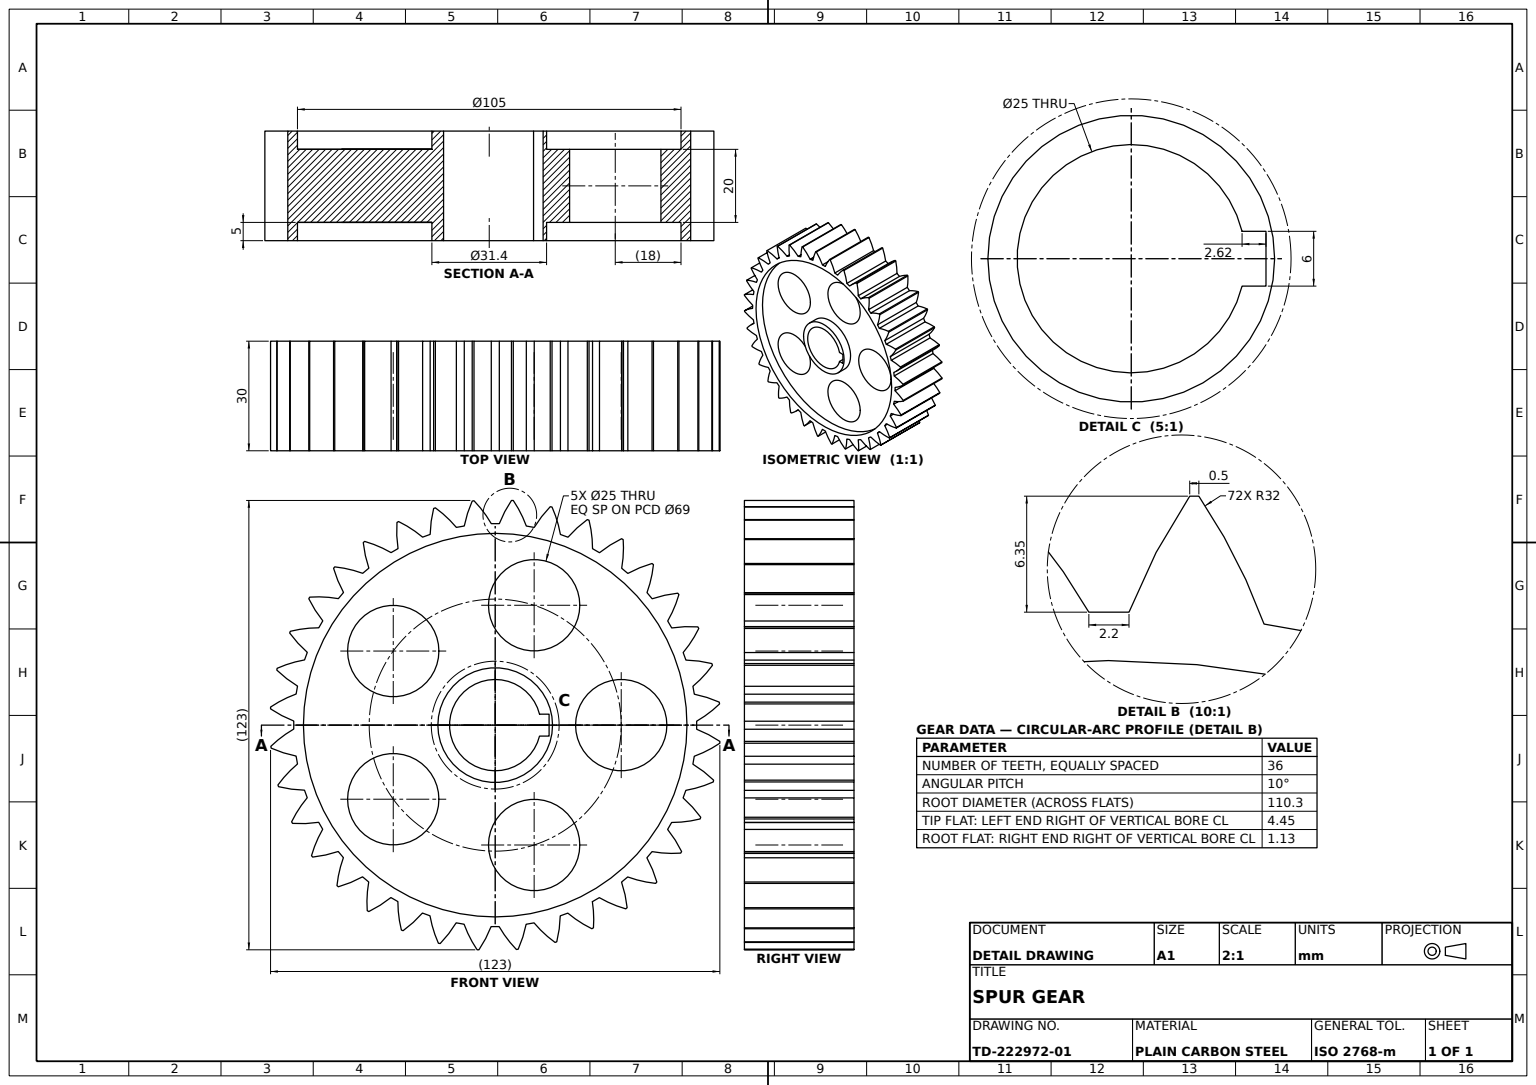
from build123d import *

# Parameters (mm, degrees)
GEAR_RIM_36T_DEPTH           = 15
SKETCH1_3_R                  = 52.5
GEAR_WEB_DEPTH               = 10
LIGHTENING_HOLES_SKETCH_R    = 12.5
LIGHTENING_HOLES_5X_18_DEPTH = 20
HUB_SKETCH_R                 = 15.7
HUB_DEPTH                    = 15
KEYED_BORE_DEPTH             = 30


with BuildPart() as part:
    # Gear Profile Sketch 36T → Gear Rim 36T (new, symmetric)
    with BuildSketch(Plane(origin=(0, 0, 0), x_dir=(1, 0, 0), z_dir=(0, 1, 0))):
        with BuildLine():
            Line((4.95, 61.5), (4.45, 61.5))
            ThreePointArc((4.45, 61.5), (2.609142561, 58.418391887), (1.125, 55.15))
            Line((1.125, 55.15), (0, 55.15))
            Line((0, 55.15), (-1.073339337, 55.15))
            ThreePointArc((-1.073339337, 55.15), (-3.245576648, 58.433413305), (-5.804564549, 61.42523529))
            Line((-5.804564549, 61.42523529), (-6.296968426, 61.338411201))
            ThreePointArc((-6.296968426, 61.338411201), (-7.574743471, 57.9839581), (-8.468788276, 54.507501778))
            Line((-8.468788276, 54.507501778), (-10.633729899, 54.125764159))
            ThreePointArc((-10.633729899, 54.125764159), (-13.343124781, 56.982089988), (-16.382760342, 59.484095888))
            Line((-16.382760342, 59.484095888), (-16.852606652, 59.313085816))
            ThreePointArc((-16.852606652, 59.313085816), (-17.528474755, 55.787711087), (-17.805256706, 52.208820698))
            Line((-17.805256706, 52.208820698), (-19.871019959, 51.456944362))
            ThreePointArc((-19.871019959, 51.456944362), (-23.03524882, 53.7993947), (-26.463174251, 55.735562333))
            Line((-26.463174251, 55.735562333), (-26.896186953, 55.485562333))
            ThreePointArc((-26.896186953, 55.485562333), (-26.949612204, 51.896382703), (-26.600721421, 48.323801019))
            Line((-26.600721421, 48.323801019), (-28.504539133, 47.22463135))
            ThreePointArc((-28.504539133, 47.22463135), (-32.02745848, 48.982032028), (-35.739518002, 50.29353192))
            Line((-35.739518002, 50.29353192), (-36.122540224, 49.972138115))
            ThreePointArc((-36.122540224, 49.972138115), (-35.551899323, 46.428208991), (-34.587936676, 42.970487099))
            Line((-34.587936676, 42.970487099), (-36.271962309, 41.557421811))
            ThreePointArc((-36.271962309, 41.557421811), (-40.04653002, 42.676375099), (-43.929934584, 43.323357989))
            Line((-43.929934584, 43.323357989), (-44.251328389, 42.940335768))
            ThreePointArc((-44.251328389, 42.940335768), (-43.073959971, 39.549337643), (-41.524214977, 36.311536673))
            Line((-41.524214977, 36.311536673), (-42.937280265, 34.627511039))
            ThreePointArc((-42.937280265, 34.627511039), (-46.84880801, 35.074018108), (-50.785562333, 35.036825749))
            Line((-50.785562333, 35.036825749), (-51.035562333, 34.603813047))
            ThreePointArc((-51.035562333, 34.603813047), (-49.287240142, 31.468779683), (-47.198801019, 28.549278579))
            Line((-47.198801019, 28.549278579), (-48.297970687, 26.645460867))
            ThreePointArc((-48.297970687, 26.645460867), (-52.227608676, 26.405954826), (-56.098096469, 25.685717287))
            Line((-56.098096469, 25.685717287), (-56.269106541, 25.215870977))
            ThreePointArc((-56.269106541, 25.215870977), (-54.002952462, 22.432058777), (-51.439275375, 19.919565103))
            Line((-51.439275375, 19.919565103), (-52.19115171, 17.853801849))
            ThreePointArc((-52.19115171, 17.853801849), (-56.01949988, 16.935559967), (-59.706118331, 15.554161304))
            Line((-59.706118331, 15.554161304), (-59.79294242, 15.061757427))
            ThreePointArc((-59.79294242, 15.061757427), (-57.077812398, 12.713751116), (-54.116793379, 10.68460572))
            Line((-54.116793379, 10.68460572), (-54.498530999, 8.519664097))
            ThreePointArc((-54.498530999, 8.519664097), (-58.109266928, 6.950586689), (-61.5, 4.95))
            Line((-61.5, 4.95), (-61.5, 4.45))
            ThreePointArc((-61.5, 4.45), (-58.418391887, 2.609142561), (-55.15, 1.125))
            Line((-55.15, 1.125), (-55.15, -1.073339337))
            ThreePointArc((-55.15, -1.073339337), (-58.433413305, -3.245576648), (-61.42523529, -5.804564549))
            Line((-61.42523529, -5.804564549), (-61.338411201, -6.296968426))
            ThreePointArc((-61.338411201, -6.296968426), (-57.9839581, -7.574743471), (-54.507501778, -8.468788276))
            Line((-54.507501778, -8.468788276), (-54.125764159, -10.633729899))
            ThreePointArc((-54.125764159, -10.633729899), (-56.982089988, -13.343124781), (-59.484095888, -16.382760342))
            Line((-59.484095888, -16.382760342), (-59.313085816, -16.852606652))
            ThreePointArc((-59.313085816, -16.852606652), (-55.787711087, -17.528474755), (-52.208820698, -17.805256706))
            Line((-52.208820698, -17.805256706), (-51.456944362, -19.871019959))
            ThreePointArc((-51.456944362, -19.871019959), (-53.7993947, -23.03524882), (-55.735562333, -26.463174251))
            Line((-55.735562333, -26.463174251), (-55.485562333, -26.896186953))
            ThreePointArc((-55.485562333, -26.896186953), (-51.896382703, -26.949612204), (-48.323801019, -26.600721421))
            Line((-48.323801019, -26.600721421), (-47.22463135, -28.504539133))
            ThreePointArc((-47.22463135, -28.504539133), (-48.982032028, -32.02745848), (-50.29353192, -35.739518002))
            Line((-50.29353192, -35.739518002), (-49.972138115, -36.122540224))
            ThreePointArc((-49.972138115, -36.122540224), (-46.428208991, -35.551899323), (-42.970487099, -34.587936676))
            Line((-42.970487099, -34.587936676), (-41.557421811, -36.271962309))
            ThreePointArc((-41.557421811, -36.271962309), (-42.676375099, -40.04653002), (-43.323357989, -43.929934584))
            Line((-43.323357989, -43.929934584), (-42.940335768, -44.251328389))
            ThreePointArc((-42.940335768, -44.251328389), (-39.549337643, -43.073959971), (-36.311536673, -41.524214977))
            Line((-36.311536673, -41.524214977), (-34.627511039, -42.937280265))
            ThreePointArc((-34.627511039, -42.937280265), (-35.074018108, -46.84880801), (-35.036825749, -50.785562333))
            Line((-35.036825749, -50.785562333), (-34.603813047, -51.035562333))
            ThreePointArc((-34.603813047, -51.035562333), (-31.468779683, -49.287240142), (-28.549278579, -47.198801019))
            Line((-28.549278579, -47.198801019), (-26.645460867, -48.297970687))
            ThreePointArc((-26.645460867, -48.297970687), (-26.405954826, -52.227608676), (-25.685717287, -56.098096469))
            Line((-25.685717287, -56.098096469), (-25.215870977, -56.269106541))
            ThreePointArc((-25.215870977, -56.269106541), (-22.432058777, -54.002952462), (-19.919565103, -51.439275375))
            Line((-19.919565103, -51.439275375), (-17.853801849, -52.19115171))
            ThreePointArc((-17.853801849, -52.19115171), (-16.935559967, -56.01949988), (-15.554161304, -59.706118331))
            Line((-15.554161304, -59.706118331), (-15.061757427, -59.79294242))
            ThreePointArc((-15.061757427, -59.79294242), (-12.713751116, -57.077812398), (-10.68460572, -54.116793379))
            Line((-10.68460572, -54.116793379), (-8.519664097, -54.498530999))
            ThreePointArc((-8.519664097, -54.498530999), (-6.950586689, -58.109266928), (-4.95, -61.5))
            Line((-4.95, -61.5), (-4.45, -61.5))
            ThreePointArc((-4.45, -61.5), (-2.609142561, -58.418391887), (-1.125, -55.15))
            Line((-1.125, -55.15), (1.073339337, -55.15))
            ThreePointArc((1.073339337, -55.15), (3.245576648, -58.433413305), (5.804564549, -61.42523529))
            Line((5.804564549, -61.42523529), (6.296968426, -61.338411201))
            ThreePointArc((6.296968426, -61.338411201), (7.574743471, -57.9839581), (8.468788276, -54.507501778))
            Line((8.468788276, -54.507501778), (10.633729899, -54.125764159))
            ThreePointArc((10.633729899, -54.125764159), (13.343124781, -56.982089988), (16.382760342, -59.484095888))
            Line((16.382760342, -59.484095888), (16.852606652, -59.313085816))
            ThreePointArc((16.852606652, -59.313085816), (17.528474755, -55.787711087), (17.805256706, -52.208820698))
            Line((17.805256706, -52.208820698), (19.871019959, -51.456944362))
            ThreePointArc((19.871019959, -51.456944362), (23.03524882, -53.7993947), (26.463174251, -55.735562333))
            Line((26.463174251, -55.735562333), (26.896186953, -55.485562333))
            ThreePointArc((26.896186953, -55.485562333), (26.949612204, -51.896382703), (26.600721421, -48.323801019))
            Line((26.600721421, -48.323801019), (28.504539133, -47.22463135))
            ThreePointArc((28.504539133, -47.22463135), (32.02745848, -48.982032028), (35.739518002, -50.29353192))
            Line((35.739518002, -50.29353192), (36.122540224, -49.972138115))
            ThreePointArc((36.122540224, -49.972138115), (35.551899323, -46.428208991), (34.587936676, -42.970487099))
            Line((34.587936676, -42.970487099), (36.271962309, -41.557421811))
            ThreePointArc((36.271962309, -41.557421811), (40.04653002, -42.676375099), (43.929934584, -43.323357989))
            Line((43.929934584, -43.323357989), (44.251328389, -42.940335768))
            ThreePointArc((44.251328389, -42.940335768), (43.073959971, -39.549337643), (41.524214977, -36.311536673))
            Line((41.524214977, -36.311536673), (42.937280265, -34.627511039))
            ThreePointArc((42.937280265, -34.627511039), (46.84880801, -35.074018108), (50.785562333, -35.036825749))
            Line((50.785562333, -35.036825749), (51.035562333, -34.603813047))
            ThreePointArc((51.035562333, -34.603813047), (49.287240142, -31.468779683), (47.198801019, -28.549278579))
            Line((47.198801019, -28.549278579), (48.297970687, -26.645460867))
            ThreePointArc((48.297970687, -26.645460867), (52.227608676, -26.405954826), (56.098096469, -25.685717287))
            Line((56.098096469, -25.685717287), (56.269106541, -25.215870977))
            ThreePointArc((56.269106541, -25.215870977), (54.002952462, -22.432058777), (51.439275375, -19.919565103))
            Line((51.439275375, -19.919565103), (52.19115171, -17.853801849))
            ThreePointArc((52.19115171, -17.853801849), (56.01949988, -16.935559967), (59.706118331, -15.554161304))
            Line((59.706118331, -15.554161304), (59.79294242, -15.061757427))
            ThreePointArc((59.79294242, -15.061757427), (57.077812398, -12.713751116), (54.116793379, -10.68460572))
            Line((54.116793379, -10.68460572), (54.498530999, -8.519664097))
            ThreePointArc((54.498530999, -8.519664097), (58.109266928, -6.950586689), (61.5, -4.95))
            Line((61.5, -4.95), (61.5, -4.45))
            ThreePointArc((61.5, -4.45), (58.418391887, -2.609142561), (55.15, -1.125))
            Line((55.15, -1.125), (55.15, 1.073339337))
            ThreePointArc((55.15, 1.073339337), (58.433413305, 3.245576648), (61.42523529, 5.804564549))
            Line((61.42523529, 5.804564549), (61.338411201, 6.296968426))
            ThreePointArc((61.338411201, 6.296968426), (57.9839581, 7.574743471), (54.507501778, 8.468788276))
            Line((54.507501778, 8.468788276), (54.125764159, 10.633729899))
            ThreePointArc((54.125764159, 10.633729899), (56.982089988, 13.343124781), (59.484095888, 16.382760342))
            Line((59.484095888, 16.382760342), (59.313085816, 16.852606652))
            ThreePointArc((59.313085816, 16.852606652), (55.787711087, 17.528474755), (52.208820698, 17.805256706))
            Line((52.208820698, 17.805256706), (51.456944362, 19.871019959))
            ThreePointArc((51.456944362, 19.871019959), (53.7993947, 23.03524882), (55.735562333, 26.463174251))
            Line((55.735562333, 26.463174251), (55.485562333, 26.896186953))
            ThreePointArc((55.485562333, 26.896186953), (51.896382703, 26.949612204), (48.323801019, 26.600721421))
            Line((48.323801019, 26.600721421), (47.22463135, 28.504539133))
            ThreePointArc((47.22463135, 28.504539133), (48.982032028, 32.02745848), (50.29353192, 35.739518002))
            Line((50.29353192, 35.739518002), (49.972138115, 36.122540224))
            ThreePointArc((49.972138115, 36.122540224), (46.428208991, 35.551899323), (42.970487099, 34.587936676))
            Line((42.970487099, 34.587936676), (41.557421811, 36.271962309))
            ThreePointArc((41.557421811, 36.271962309), (42.676375099, 40.04653002), (43.323357989, 43.929934584))
            Line((43.323357989, 43.929934584), (42.940335768, 44.251328389))
            ThreePointArc((42.940335768, 44.251328389), (39.549337643, 43.073959971), (36.311536673, 41.524214977))
            Line((36.311536673, 41.524214977), (34.627511039, 42.937280265))
            ThreePointArc((34.627511039, 42.937280265), (35.074018108, 46.84880801), (35.036825749, 50.785562333))
            Line((35.036825749, 50.785562333), (34.603813047, 51.035562333))
            ThreePointArc((34.603813047, 51.035562333), (31.468779683, 49.287240142), (28.549278579, 47.198801019))
            Line((28.549278579, 47.198801019), (26.645460867, 48.297970687))
            ThreePointArc((26.645460867, 48.297970687), (26.405954826, 52.227608676), (25.685717287, 56.098096469))
            Line((25.685717287, 56.098096469), (25.215870977, 56.269106541))
            ThreePointArc((25.215870977, 56.269106541), (22.432058777, 54.002952462), (19.919565103, 51.439275375))
            Line((19.919565103, 51.439275375), (17.853801849, 52.19115171))
            ThreePointArc((17.853801849, 52.19115171), (16.935559967, 56.01949988), (15.554161304, 59.706118331))
            Line((15.554161304, 59.706118331), (15.061757427, 59.79294242))
            ThreePointArc((15.061757427, 59.79294242), (12.713751116, 57.077812398), (10.68460572, 54.116793379))
            Line((10.68460572, 54.116793379), (8.519664097, 54.498530999))
            ThreePointArc((8.519664097, 54.498530999), (6.950586689, 58.109266928), (4.95, 61.5))
        make_face()
        with BuildLine():
            ThreePointArc((9.340780487, 51.662363669), (40.290451571, 33.659018289), (52.5, 0))
            ThreePointArc((52.5, 0), (-30.233163158, -42.920925497), (-17.679270304, 49.433727368))
            ThreePointArc((-17.679270304, 49.433727368), (-13.303562118, 50.786467046), (-8.826605791, 51.752691043))
            ThreePointArc((-8.826605791, 51.752691043), (0.261024258, 52.499351104), (9.340780487, 51.662363669))
        make_face(mode=Mode.SUBTRACT)
    extrude(amount=GEAR_RIM_36T_DEPTH, both=True)

    # Sketch1_3 → Gear Web (add, symmetric)
    with BuildSketch(Plane(origin=(0, 0, 0), x_dir=(1, 0, 0), z_dir=(0, 1, 0))):
        with Locations(Location((0, 0, 0), (0, 0, 270))):
            Circle(SKETCH1_3_R)
    extrude(amount=GEAR_WEB_DEPTH, both=True)

    # Lightening Holes Sketch → Lightening Holes 5x_18 (cut)
    with BuildSketch(Plane(origin=(0, 10, 0), x_dir=(1, 0, 0), z_dir=(0, 1, 0))):
        with Locations(Location((0, 34.5, 0), (0, 0, 270))):
            Circle(LIGHTENING_HOLES_SKETCH_R)
        with Locations(Location((32.811449812, 10.661086306, 0), (0, 0, 270))):
            Circle(LIGHTENING_HOLES_SKETCH_R)
        with Locations(Location((20.278591204, -27.911086306, 0), (0, 0, 270))):
            Circle(LIGHTENING_HOLES_SKETCH_R)
        with Locations(Location((-20.278591204, -27.911086306, 0), (0, 0, 270))):
            Circle(LIGHTENING_HOLES_SKETCH_R)
        with Locations(Location((-32.811449812, 10.661086306, 0), (0, 0, 270))):
            Circle(LIGHTENING_HOLES_SKETCH_R)
    extrude(amount=-LIGHTENING_HOLES_5X_18_DEPTH, mode=Mode.SUBTRACT)

    # Hub Sketch → Hub (add, symmetric)
    with BuildSketch(Plane(origin=(0, 0, 0), x_dir=(1, 0, 0), z_dir=(0, 1, 0))):
        with Locations(Location((0, 0, 0), (0, 0, 270))):
            Circle(HUB_SKETCH_R)
        with BuildLine():
            Line((-3, 14.75362242), (3, 14.75362242))
            Line((3, 14.75362242), (3, 12.1346611))
            ThreePointArc((3, 12.1346611), (0, -12.5), (-3, 12.1346611))
            Line((-3, 12.1346611), (-3, 14.75362242))
        make_face(mode=Mode.SUBTRACT)
    extrude(amount=HUB_DEPTH, both=True)

    # Keyed Bore Sketch → Keyed Bore (cut)
    with BuildSketch(Plane(origin=(0, 15, 0), x_dir=(1, 0, 0), z_dir=(0, 1, 0))):
        with BuildLine():
            Line((3, 12.1346611), (3, 14.75362242))
            Line((3, 14.75362242), (-3, 14.75362242))
            Line((-3, 14.75362242), (-3, 12.1346611))
            ThreePointArc((-3, 12.1346611), (0, -12.5), (3, 12.1346611))
        make_face()
    extrude(amount=-KEYED_BORE_DEPTH, mode=Mode.SUBTRACT)


solid = part.part
